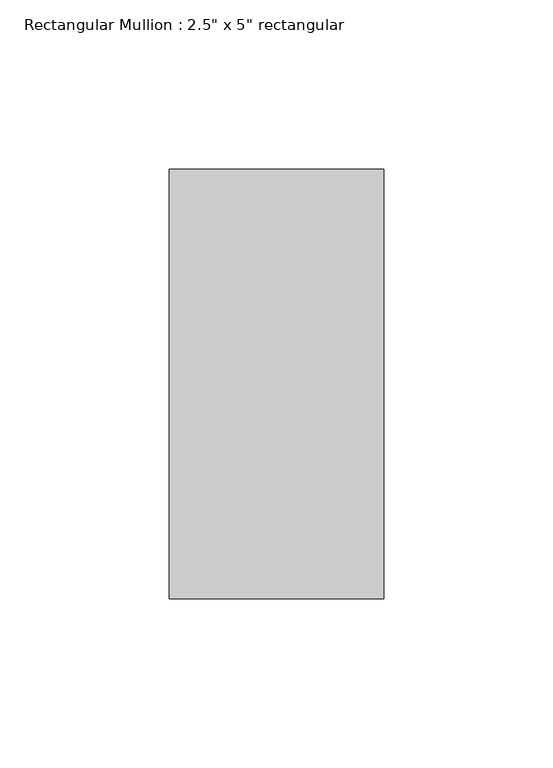
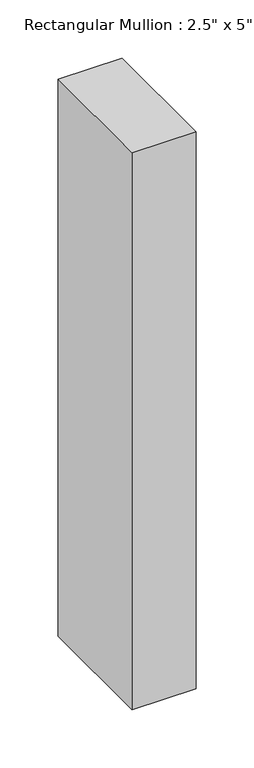
"""IFC4 building model written with IfcOpenShell, lengths in millimetres: member geometry."""

from ifc_helpers import new_model, si_unit, frame, origin, place, context, project, spatial, polyline, outline, extrude, source, transform, mapped, element, save


def member_ea55af56(model_context):
    return source(origin(), model_context, "Body", "SweptSolid", [
        extrude(outline(polyline([(0.0, 63.5), (0.0, -63.5), (-63.5, -63.5), (-63.5, 63.5), (0.0, 63.5)])), frame((0.0, 0.0, -583.8967564), z_axis=(0.0, 0.0, 1.0), x_axis=(1.0, 0.0, 0.0)), (0.0, 0.0, 1.0), 583.8967564),
    ])


if __name__ == "__main__":
    model = new_model("IFC4")
    model_context = context("Model", 3, world=origin())
    ifc_project = project(units=[si_unit("LENGTHUNIT", "METRE", prefix="MILLI")], contexts=[model_context])
    site = spatial("IfcSite", under=ifc_project)
    building = spatial("IfcBuilding", under=site)
    placement = place(None, origin())
    member_shape = member_ea55af56(model_context)
    element("IfcMember", 1, ObjectType="Rectangular Mullion : 2.5\" x 5\" rectangular", at=placement, inside=building, context=model_context, shape_type="MappedRepresentation", body=[
        mapped(member_shape, transform((0.0, 0.0, 0.0), x_axis=(1.0, 0.0, 0.0), y_axis=(0.0, 1.0, 0.0), z_axis=(0.0, 0.0, 1.0))),
    ])
    save(model, "model.ifc")

# Revit data of these elements
# Type "Rectangular Mullion : 2.5\" x 5\" rectangular"
#   built-in parameter 1007304 = 0.416667 (stored number, unit not read)
#   built-in parameter 1007301 = 0.104167 (stored number, unit not read)
#   built-in parameter 1007300 = 0.104167 (stored number, unit not read)
# Element 1 (IfcMember, "Rectangular Mullion : 2.5\" x 5\" rectangular")
#   Materials on its faces: "Aluminum"
# Materials
#   "Aluminum": class "Metal", colour RGB 247 247 247, transparency 0, Description = "Aluminum 6061", Cost = 0
